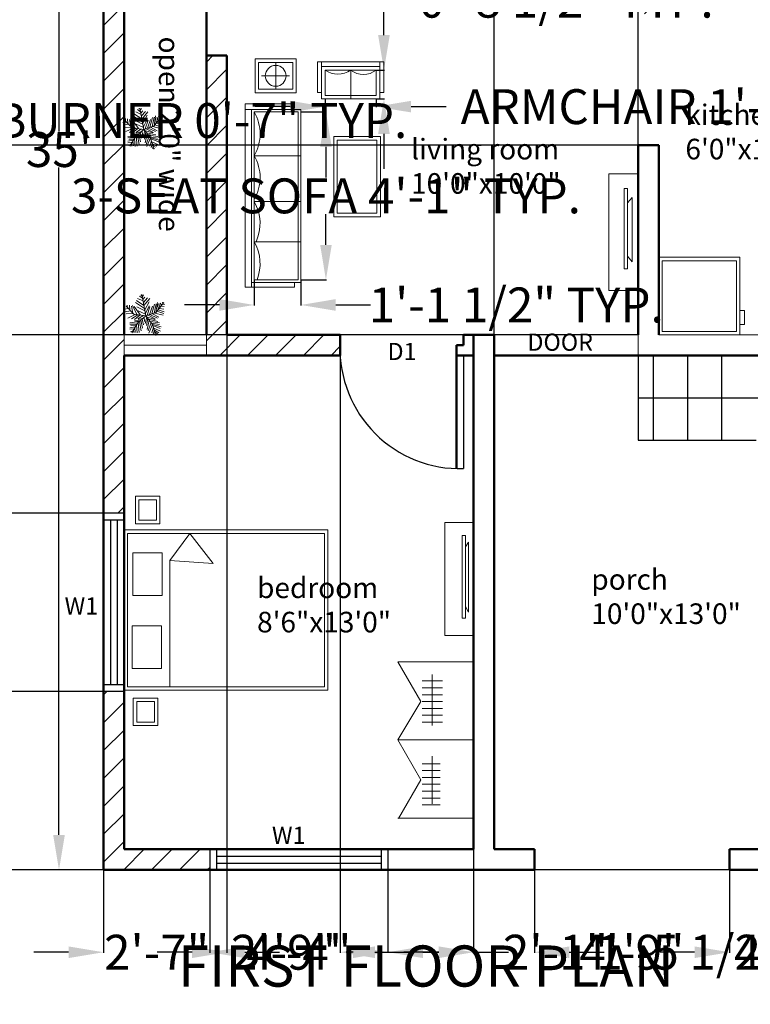
# Model space of a CAD drawing. Units: inches. Extents: x 21 to 3450, y 4 to 2137.
# Tile 12 of 14: x 3122 to 3335, y 1057 to 1344. Entities that reach past the tile are written whole.
import ezdxf

# ---------------------------------------------------------------- set-up
doc = ezdxf.new("R2010")
doc.units = ezdxf.units.IN
doc.header["$MEASUREMENT"] = 0
for name, color, linetype, lineweight in [('A-ANNO-DIMS', 2, 'Continuous', 18), ('A-ANNO-TEXT', 7, 'Continuous', 18), ('A-AREA-IDEN', 3, 'Continuous', 18), ('A-DOOR', 4, 'Continuous', 25), ('A-FLOR-FIXT', 9, 'Continuous', 18), ('A-FLOR-STRS', 2, 'Continuous', 25), ('A-FURN', 8, 'Continuous', 18), ('A-GLAZ', 3, 'Continuous', 25), ('A-WALL', 7, 'Continuous', 50), ('A-WALL-PATT', 8, 'Continuous', 13), ('L-PLNT', 94, 'Continuous', 13)]:
    doc.layers.add(name, color=color, linetype=linetype, lineweight=lineweight)
doc.styles.get("Standard").update_dxf_attribs({"font": 'arial.ttf'})
doc.dimstyles.get("Standard").update_dxf_attribs({"dimtxt": 10.18, "dimasz": 10.18, "dimexe": 0.18, "dimexo": 0.0625, "dimgap": 0.09, "dimtad": 0, "dimtih": 1, "dimtoh": 1, "dimdec": 0, "dimzin": 0, "dimdsep": 46, "dimlunit": 3, "dimtxsty": 'Standard', "dimcen": 0.09, "dimadec": 0, "dimazin": 0, "dimtfac": 1, "dimtdec": 0, "dimtofl": 0, "dimtmove": 0, "dimatfit": 3, "dimfxl": 1, "dimtolj": 1, "dimtzin": 0, "dimarcsym": 0})

# ---------------------------------------------------------------- blocks, each defined once
blk = doc.blocks.new('*U6')
for p, q in [((-8.737, 47.138), (-17.069, 52.711)), ((-10.186, 53.64), (-13.084, 55.962)), ((0, 0), (-10.5, 57)), ((-9.099, 51.782), (-6.563, 55.962)), ((-48.585, 21.131), (-49.309, 29.026)), ((-43.513, 28.561), (-42.427, 15.558)), ((-38.442, 26.239), (-34.819, 7.663)), ((-35.544, 28.097), (-24.314, 3.947)), ((-3.665, 19.273), (-27.574, 35.527)), ((-5.114, 28.097), (-24.676, 40.636)), ((-7.288, 39.707), (-21.778, 46.673)), ((-7.65, 43.423), (-2.578, 49.46)), ((-5.839, 35.992), (4.667, 48.067)), ((-5.114, 27.632), (10.463, 46.673)), ((-2.941, 16.486), (8.652, 37.85)), ((-1.129, 6.734), (9.014, 26.704)), ((10.101, 3.483), (17.708, 26.239)), ((16.259, 5.805), (23.142, 31.348)), ((22.055, 7.198), (27.489, 32.277)), ((27, 9), (48, 36)), ((27.127, 9.056), (31.112, 35.992)), ((31.836, 30.883), (32.561, 16.486)), ((35.096, 32.741), (37.27, 22.524)), ((38.719, 34.134), (41.979, 28.561)), ((43.791, 29.954), (51.036, 30.883)), ((44.153, 36.456), (45.239, 32.741)), ((-47.498, 19.737), (-55.83, 18.344)), ((-40.615, 13.7), (-55.105, 10.913)), ((-31.5, 4.5), (-52.5, 25.5)), ((-33.37, 6.269), (-52.207, 5.34)), ((-28.299, 3.483), (-47.86, -5.805)), ((-21.416, 3.018), (-38.079, -8.128)), ((0, 0), (-31.5, 4.5)), ((-14.533, 2.09), (-30.834, 25.31)), ((-15.982, 2.09), (-30.11, -9.521)), ((-24.314, 23.917), (-2.941, 13.7)), ((0, 0), (-22.5, -19.5)), ((-6.563, 1.161), (-21.416, -8.128)), ((-20.691, 13.7), (-1.129, 4.876)), ((0, 0), (27, 9)), ((0, 0), (18, -22.5)), ((3.942, 1.625), (11.187, 24.381)), ((6.478, 1.625), (26.04, -8.592)), ((11.187, 3.483), (30.749, -5.805)), ((18.07, 5.805), (35.096, -3.483)), ((24.229, 7.663), (46.688, 1.625)), ((29.662, 12.307), (48.137, 6.269)), ((33.285, 16.486), (48.862, 10.913)), ((36.183, 19.737), (48.137, 17.88)), ((40.53, 25.775), (48.862, 24.846)), ((-17.431, -15.094), (-42.789, -18.809)), ((-24.314, -21.596), (-42.427, -22.06)), ((-26.849, -26.24), (-40.253, -25.775)), ((-22.5, -19.5), (-37.5, -45)), ((-15.257, -12.772), (-30.11, -12.772)), ((-25.038, -23.918), (-22.865, -45.281)), ((-20.691, -18.345), (-17.793, -44.352)), ((-6.563, -5.805), (-19.967, -9.985)), ((-17.069, -15.094), (-12.721, -40.172)), ((-13.446, -11.378), (-8.737, -32.741)), ((-9.461, -8.592), (-6.201, -23.453)), ((-4.752, -3.483), (-3.665, -14.629)), ((2.493, -3.019), (-1.491, -20.202)), ((1.769, -2.555), (24.229, -9.521)), ((5.029, -6.27), (2.131, -25.775)), ((9.014, -11.378), (3.58, -35.992)), ((14.085, -16.951), (6.478, -40.172)), ((7.565, -9.056), (32.198, -14.629)), ((18.07, -22.524), (8.289, -45.745)), ((12.274, -15.094), (36.907, -18.809)), ((16.259, -19.738), (36.183, -22.989)), ((18, -22.5), (27, -52.5)), ((18.433, -22.524), (40.53, -29.026)), ((19.157, -25.311), (38.719, -33.206)), ((-28.299, -29.026), (-42.789, -31.348)), ((-30.834, -34.135), (-42.427, -35.528)), ((-34.457, -39.708), (-40.978, -42.494)), ((-32.646, -36.921), (-31.921, -44.352)), ((-29.023, -30.884), (-27.936, -43.887)), ((20.244, -30.419), (15.897, -44.816)), ((22.78, -37.85), (19.519, -48.532)), ((21.331, -32.741), (39.081, -40.636)), ((22.78, -38.314), (34.372, -44.816)), ((24.591, -45.745), (23.142, -50.854)), ((24.591, -43.423), (30.749, -47.603)), ((26.764, -49.925), (28.213, -50.854))]:
    blk.add_line(p, q)
blk = doc.blocks.new('*D10')
at = {"layer": 'A-ANNO-DIMS', "color": 0, "lineweight": -2, "transparency": 16777216}
for p, q in [((3146.55, 1515.83), (3133.43, 1515.83)), ((3133.61, 1505.65), (3133.61, 1311.09)), ((3133.61, 1105.95), (3133.61, 1300.51)), ((3329.19, 1095.77), (3133.43, 1095.77))]:
    blk.add_line(p, q, dxfattribs=at)
at = {"layer": 'A-ANNO-DIMS', "color": 0, "transparency": 16777216}
for points in [[(3131.91, 1505.65), (3135.31, 1505.65), (3133.61, 1515.83)], [(3131.91, 1105.95), (3135.31, 1105.95), (3133.61, 1095.77)]]:
    blk.add_solid(points, dxfattribs=at)
at = {"layer": 'Defpoints', "color": 0, "transparency": 16777216}
for p in [(3146.61, 1515.83), (3133.61, 1095.77), (3329.26, 1095.77)]:
    blk.add_point(p, dxfattribs=at)
at = {"layer": 'A-ANNO-DIMS', "color": 0, "transparency": 16777216, "insert": (3133.61, 1305.8), "char_height": 10.18, "attachment_point": 5}
blk.add_mtext("\\A1;35'", dxfattribs=at)
blk = doc.blocks.new('DOOR-35IN')
blk.add_line((36, 33.01), (36, 0.01))
blk.add_arc((35, 35.01), 35.01, 178.3634, 271.6366)
blk = doc.blocks.new('SOFA-3SEAT')
blk.add_line((0, 36.17), (13.59, 36.17))
blk.add_lwpolyline([(0, 48.92), (12.82, 48.92), (12.82, 0), (0, 0)], close=True)
for centre in [(-11.01, 42.54), (-11.01, 29.79)]:
    blk.add_arc(centre, 12.72, 329.9119, 30.0881)
blk = doc.blocks.new('ARMCHAIR')
blk.add_line((7.48, 8.43), (7.48, 0))
blk.add_lwpolyline([(0, 8.43), (14.95, 8.43), (14.95, 1), (0, 1)], close=True)
for centre, radius, start, end in [((3.74, 13.52), 6.31, 233.6798, 306.3202), ((11.21, 13.17), 6.03, 231.7288, 308.2712)]:
    blk.add_arc(centre, radius, start, end)
blk = doc.blocks.new('*D28')
at = {"layer": 'A-ANNO-DIMS', "color": 0, "lineweight": -2, "transparency": 16777216}
for p, q in [((3204.23, 1316.74), (3211.68, 1316.74)), ((3211.5, 1306.56), (3211.5, 1297.64)), ((3211.5, 1278), (3211.5, 1286.92)), ((3204.23, 1267.82), (3211.68, 1267.82))]:
    blk.add_line(p, q, dxfattribs=at)
at = {"layer": 'A-ANNO-DIMS', "color": 0, "transparency": 16777216}
for points in [[(3209.81, 1306.56), (3213.2, 1306.56), (3211.5, 1316.74)], [(3209.81, 1278), (3213.2, 1278), (3211.5, 1267.82)]]:
    blk.add_solid(points, dxfattribs=at)
at = {"layer": 'Defpoints', "color": 0, "transparency": 16777216}
for p in [(3204.17, 1316.74), (3211.5, 1316.74), (3204.17, 1267.82)]:
    blk.add_point(p, dxfattribs=at)
at = {"layer": 'A-ANNO-DIMS', "color": 0, "transparency": 16777216, "insert": (3211.5, 1292.28), "char_height": 10.18, "attachment_point": 5}
blk.add_mtext('\\A1;3-SEAT SOFA 4\'-1" TYP.', dxfattribs=at)
blk = doc.blocks.new('*D29')
at = {"layer": 'A-ANNO-DIMS', "color": 0, "lineweight": -2, "transparency": 16777216}
for p, q in [((3190.58, 1267.76), (3190.58, 1260.3)), ((3204.17, 1267.76), (3204.17, 1260.3)), ((3180.4, 1260.48), (3170.22, 1260.48)), ((3214.35, 1260.48), (3224.53, 1260.48))]:
    blk.add_line(p, q, dxfattribs=at)
at = {"layer": 'A-ANNO-DIMS', "color": 0, "transparency": 16777216}
for points in [[(3180.4, 1262.18), (3180.4, 1258.78), (3190.58, 1260.48)], [(3214.35, 1262.18), (3214.35, 1258.78), (3204.17, 1260.48)]]:
    blk.add_solid(points, dxfattribs=at)
at = {"layer": 'Defpoints', "color": 0, "transparency": 16777216}
for p in [(3190.58, 1267.82), (3204.17, 1267.82), (3204.17, 1260.48)]:
    blk.add_point(p, dxfattribs=at)
at = {"layer": 'A-ANNO-DIMS', "color": 0, "transparency": 16777216, "insert": (3267.02, 1260.48), "char_height": 10.18, "attachment_point": 5}
blk.add_mtext('\\A1;1\'-1 1/2" TYP.', dxfattribs=at)
blk = doc.blocks.new('*D30')
at = {"layer": 'A-ANNO-DIMS', "color": 0, "lineweight": -2, "transparency": 16777216}
for p, q in [((3201.06, 1318.3), (3190.88, 1318.3)), ((3211.24, 1320.48), (3211.24, 1318.12)), ((3226.19, 1320.48), (3226.19, 1318.12)), ((3236.37, 1318.3), (3246.55, 1318.3))]:
    blk.add_line(p, q, dxfattribs=at)
at = {"layer": 'A-ANNO-DIMS', "color": 0, "transparency": 16777216}
for points in [[(3201.06, 1320), (3201.06, 1316.61), (3211.24, 1318.3)], [(3236.37, 1320), (3236.37, 1316.61), (3226.19, 1318.3)]]:
    blk.add_solid(points, dxfattribs=at)
at = {"layer": 'Defpoints', "color": 0, "transparency": 16777216}
for p in [(3211.24, 1320.54), (3226.19, 1320.54), (3226.19, 1318.3)]:
    blk.add_point(p, dxfattribs=at)
at = {"layer": 'A-ANNO-DIMS', "color": 0, "transparency": 16777216, "insert": (3317.86, 1318.3), "char_height": 10.18, "attachment_point": 5}
blk.add_mtext('\\A1;ARMCHAIR 1\'-3" TYP.', dxfattribs=at)
blk = doc.blocks.new('*D31')
at = {"layer": 'A-ANNO-DIMS', "color": 0, "lineweight": -2, "transparency": 16777216}
for p, q in [((3228.43, 1339.16), (3228.43, 1349.34)), ((3228.43, 1349.34), (3238.61, 1349.34)), ((3226.25, 1328.98), (3228.61, 1328.98)), ((3226.25, 1320.54), (3228.61, 1320.54)), ((3228.43, 1310.36), (3228.43, 1300.18))]:
    blk.add_line(p, q, dxfattribs=at)
at = {"layer": 'A-ANNO-DIMS', "color": 0, "transparency": 16777216}
for points in [[(3226.74, 1339.16), (3230.13, 1339.16), (3228.43, 1328.98)], [(3226.74, 1310.36), (3230.13, 1310.36), (3228.43, 1320.54)]]:
    blk.add_solid(points, dxfattribs=at)
at = {"layer": 'Defpoints', "color": 0, "transparency": 16777216}
for p in [(3226.19, 1328.98), (3228.43, 1328.98), (3226.19, 1320.54)]:
    blk.add_point(p, dxfattribs=at)
at = {"layer": 'A-ANNO-DIMS', "color": 0, "transparency": 16777216, "insert": (3281.59, 1349.34), "char_height": 10.18, "attachment_point": 5}
blk.add_mtext('\\A1;0\'-8 1/2" TYP.', dxfattribs=at)
blk = doc.blocks.new('*D32')
at = {"layer": 'A-ANNO-DIMS', "color": 0, "lineweight": -2, "transparency": 16777216}
for p, q in [((3035.54, 1315.23), (3035.54, 1314.07)), ((3042.48, 1315.23), (3042.48, 1314.07)), ((3025.36, 1314.25), (3015.18, 1314.25)), ((3052.66, 1314.25), (3062.84, 1314.25))]:
    blk.add_line(p, q, dxfattribs=at)
at = {"layer": 'A-ANNO-DIMS', "color": 0, "transparency": 16777216}
for points in [[(3025.36, 1315.95), (3025.36, 1312.56), (3035.54, 1314.25)], [(3052.66, 1315.95), (3052.66, 1312.56), (3042.48, 1314.25)]]:
    blk.add_solid(points, dxfattribs=at)
at = {"layer": 'Defpoints', "color": 0, "transparency": 16777216}
for p in [(3035.54, 1315.29), (3042.48, 1315.29), (3042.48, 1314.25)]:
    blk.add_point(p, dxfattribs=at)
at = {"layer": 'A-ANNO-DIMS', "color": 0, "transparency": 16777216, "insert": (3152.02, 1314.25), "char_height": 10.18, "attachment_point": 5}
blk.add_mtext('\\A1;STOVE BURNER 0\'-7" TYP.', dxfattribs=at)
blk = doc.blocks.new('*D128')
at = {"layer": 'A-ANNO-DIMS', "color": 0, "lineweight": -2, "transparency": 16777216}
for p, q in [((3146.61, 1095.7), (3146.61, 1071.59)), ((3177.61, 1095.7), (3177.61, 1071.59)), ((3136.43, 1071.77), (3126.25, 1071.77)), ((3187.79, 1071.77), (3197.97, 1071.77))]:
    blk.add_line(p, q, dxfattribs=at)
at = {"layer": 'A-ANNO-DIMS', "color": 0, "transparency": 16777216}
for points in [[(3136.43, 1073.46), (3136.43, 1070.07), (3146.61, 1071.77)], [(3187.79, 1073.46), (3187.79, 1070.07), (3177.61, 1071.77)]]:
    blk.add_solid(points, dxfattribs=at)
at = {"layer": 'Defpoints', "color": 0, "transparency": 16777216}
for p in [(3146.61, 1095.77), (3177.61, 1095.77), (3177.61, 1071.77)]:
    blk.add_point(p, dxfattribs=at)
at = {"layer": 'A-ANNO-DIMS', "color": 0, "transparency": 16777216, "insert": (3162.11, 1071.77), "char_height": 10.18, "attachment_point": 5}
blk.add_mtext('\\A1;2\'-7"', dxfattribs=at)
blk = doc.blocks.new('*D129')
at = {"layer": 'A-ANNO-DIMS', "color": 0, "lineweight": -2, "transparency": 16777216}
for p, q in [((3177.61, 1095.7), (3177.61, 1071.59)), ((3229.61, 1095.7), (3229.61, 1071.59)), ((3187.79, 1071.77), (3189.79, 1071.77)), ((3219.43, 1071.77), (3217.44, 1071.77))]:
    blk.add_line(p, q, dxfattribs=at)
at = {"layer": 'A-ANNO-DIMS', "color": 0, "transparency": 16777216}
for points in [[(3187.79, 1073.46), (3187.79, 1070.07), (3177.61, 1071.77)], [(3219.43, 1073.46), (3219.43, 1070.07), (3229.61, 1071.77)]]:
    blk.add_solid(points, dxfattribs=at)
at = {"layer": 'Defpoints', "color": 0, "transparency": 16777216}
for p in [(3177.61, 1095.77), (3229.61, 1095.77), (3229.61, 1071.77)]:
    blk.add_point(p, dxfattribs=at)
at = {"layer": 'A-ANNO-DIMS', "color": 0, "transparency": 16777216, "insert": (3203.61, 1071.77), "char_height": 10.18, "attachment_point": 5}
blk.add_mtext('\\A1;4\'-4"', dxfattribs=at)
blk = doc.blocks.new('*D130')
at = {"layer": 'A-ANNO-DIMS', "color": 0, "lineweight": -2, "transparency": 16777216}
for p, q in [((3254.61, 1101.7), (3254.61, 1071.59)), ((3229.61, 1095.7), (3229.61, 1071.59)), ((3239.79, 1071.77), (3244.43, 1071.77)), ((3254.61, 1071.77), (3264.79, 1071.77))]:
    blk.add_line(p, q, dxfattribs=at)
at = {"layer": 'A-ANNO-DIMS', "color": 0, "transparency": 16777216}
for points in [[(3239.79, 1073.46), (3239.79, 1070.07), (3229.61, 1071.77)], [(3244.43, 1073.46), (3244.43, 1070.07), (3254.61, 1071.77)]]:
    blk.add_solid(points, dxfattribs=at)
at = {"layer": 'Defpoints', "color": 0, "transparency": 16777216}
for p in [(3254.61, 1101.77), (3229.61, 1095.77), (3254.61, 1071.77)]:
    blk.add_point(p, dxfattribs=at)
at = {"layer": 'A-ANNO-DIMS', "color": 0, "transparency": 16777216, "insert": (3278.5, 1071.77), "char_height": 10.18, "attachment_point": 5}
blk.add_mtext('\\A1;2\'-1"', dxfattribs=at)
blk = doc.blocks.new('*D131')
at = {"layer": 'A-ANNO-DIMS', "color": 0, "lineweight": -2, "transparency": 16777216}
for p, q in [((3254.61, 1101.7), (3254.61, 1071.59)), ((3272.34, 1095.7), (3272.34, 1071.59)), ((3244.43, 1071.77), (3234.25, 1071.77)), ((3282.52, 1071.77), (3292.7, 1071.77))]:
    blk.add_line(p, q, dxfattribs=at)
at = {"layer": 'A-ANNO-DIMS', "color": 0, "transparency": 16777216}
for points in [[(3244.43, 1073.46), (3244.43, 1070.07), (3254.61, 1071.77)], [(3282.52, 1073.46), (3282.52, 1070.07), (3272.34, 1071.77)]]:
    blk.add_solid(points, dxfattribs=at)
at = {"layer": 'Defpoints', "color": 0, "transparency": 16777216}
for p in [(3254.61, 1101.77), (3272.34, 1095.77), (3272.34, 1071.77)]:
    blk.add_point(p, dxfattribs=at)
at = {"layer": 'A-ANNO-DIMS', "color": 0, "transparency": 16777216, "insert": (3317.7, 1071.77), "char_height": 10.18, "attachment_point": 5}
blk.add_mtext('\\A1;1\'-5 1/2"', dxfattribs=at)
blk = doc.blocks.new('*D132')
at = {"layer": 'A-ANNO-DIMS', "color": 0, "lineweight": -2, "transparency": 16777216}
for p, q in [((3272.34, 1095.7), (3272.34, 1071.59)), ((3329.26, 1095.7), (3329.26, 1071.59)), ((3282.52, 1071.77), (3286.97, 1071.77)), ((3319.08, 1071.77), (3314.62, 1071.77))]:
    blk.add_line(p, q, dxfattribs=at)
at = {"layer": 'A-ANNO-DIMS', "color": 0, "transparency": 16777216}
for points in [[(3282.52, 1073.46), (3282.52, 1070.07), (3272.34, 1071.77)], [(3319.08, 1073.46), (3319.08, 1070.07), (3329.26, 1071.77)]]:
    blk.add_solid(points, dxfattribs=at)
at = {"layer": 'Defpoints', "color": 0, "transparency": 16777216}
for p in [(3272.34, 1095.77), (3329.26, 1095.77), (3329.26, 1071.77)]:
    blk.add_point(p, dxfattribs=at)
at = {"layer": 'A-ANNO-DIMS', "color": 0, "transparency": 16777216, "insert": (3300.8, 1071.77), "char_height": 10.18, "attachment_point": 5}
blk.add_mtext('\\A1;4\'-9"', dxfattribs=at)
blk = doc.blocks.new('*D133')
at = {"layer": 'A-ANNO-DIMS', "color": 0, "lineweight": -2, "transparency": 16777216}
for p, q in [((3329.26, 1095.7), (3329.26, 1071.59)), ((3386.61, 1095.7), (3386.61, 1071.59)), ((3319.08, 1071.77), (3308.9, 1071.77)), ((3396.79, 1071.77), (3406.97, 1071.77))]:
    blk.add_line(p, q, dxfattribs=at)
at = {"layer": 'A-ANNO-DIMS', "color": 0, "transparency": 16777216}
for points in [[(3319.08, 1073.46), (3319.08, 1070.07), (3329.26, 1071.77)], [(3396.79, 1073.46), (3396.79, 1070.07), (3386.61, 1071.77)]]:
    blk.add_solid(points, dxfattribs=at)
at = {"layer": 'Defpoints', "color": 0, "transparency": 16777216}
for p in [(3329.26, 1095.77), (3386.61, 1095.77), (3386.61, 1071.77)]:
    blk.add_point(p, dxfattribs=at)
at = {"layer": 'A-ANNO-DIMS', "color": 0, "transparency": 16777216, "insert": (3357.93, 1071.77), "char_height": 10.18, "attachment_point": 5}
blk.add_mtext('\\A1;4\'-9 1/2"', dxfattribs=at)
blk = doc.blocks.new('*D141')
at = {"layer": 'A-ANNO-DIMS', "color": 0, "lineweight": -2, "transparency": 16777216}
for p, q in [((3146.55, 1147.77), (3068.43, 1147.77)), ((3068.61, 1137.59), (3068.61, 1126.95)), ((3068.61, 1105.95), (3068.61, 1116.59)), ((3146.55, 1095.77), (3068.43, 1095.77))]:
    blk.add_line(p, q, dxfattribs=at)
at = {"layer": 'A-ANNO-DIMS', "color": 0, "transparency": 16777216}
for points in [[(3066.91, 1137.59), (3070.31, 1137.59), (3068.61, 1147.77)], [(3066.91, 1105.95), (3070.31, 1105.95), (3068.61, 1095.77)]]:
    blk.add_solid(points, dxfattribs=at)
at = {"layer": 'Defpoints', "color": 0, "transparency": 16777216}
for p in [(3068.61, 1147.77), (3146.61, 1147.77), (3146.61, 1095.77)]:
    blk.add_point(p, dxfattribs=at)
at = {"layer": 'A-ANNO-DIMS', "color": 0, "transparency": 16777216, "insert": (3068.61, 1121.77), "char_height": 10.18, "attachment_point": 5}
blk.add_mtext('\\A1;4\'-4"', dxfattribs=at)
blk = doc.blocks.new('*D142')
at = {"layer": 'A-ANNO-DIMS', "color": 0, "lineweight": -2, "transparency": 16777216}
for p, q in [((3146.55, 1199.77), (3068.43, 1199.77)), ((3068.61, 1189.59), (3068.61, 1178.95)), ((3068.61, 1157.95), (3068.61, 1168.59)), ((3146.55, 1147.77), (3068.43, 1147.77))]:
    blk.add_line(p, q, dxfattribs=at)
at = {"layer": 'A-ANNO-DIMS', "color": 0, "transparency": 16777216}
for points in [[(3066.91, 1189.59), (3070.31, 1189.59), (3068.61, 1199.77)], [(3066.91, 1157.95), (3070.31, 1157.95), (3068.61, 1147.77)]]:
    blk.add_solid(points, dxfattribs=at)
at = {"layer": 'Defpoints', "color": 0, "transparency": 16777216}
for p in [(3068.61, 1199.77), (3146.61, 1199.77), (3146.61, 1147.77)]:
    blk.add_point(p, dxfattribs=at)
at = {"layer": 'A-ANNO-DIMS', "color": 0, "transparency": 16777216, "insert": (3068.61, 1173.77), "char_height": 10.18, "attachment_point": 5}
blk.add_mtext('\\A1;4\'-4"', dxfattribs=at)
blk = doc.blocks.new('*D144')
at = {"layer": 'A-ANNO-DIMS', "color": 0, "lineweight": -2, "transparency": 16777216}
for p, q in [((3182.61, 1251.7), (3182.61, 1071.59)), ((3215.61, 1251.7), (3215.61, 1071.59)), ((3172.43, 1071.77), (3162.25, 1071.77)), ((3225.79, 1071.77), (3235.97, 1071.77))]:
    blk.add_line(p, q, dxfattribs=at)
at = {"layer": 'A-ANNO-DIMS', "color": 0, "transparency": 16777216}
for points in [[(3172.43, 1073.46), (3172.43, 1070.07), (3182.61, 1071.77)], [(3225.79, 1073.46), (3225.79, 1070.07), (3215.61, 1071.77)]]:
    blk.add_solid(points, dxfattribs=at)
at = {"layer": 'Defpoints', "color": 0, "transparency": 16777216}
for p in [(3182.61, 1251.77), (3215.61, 1251.77), (3215.61, 1071.77)]:
    blk.add_point(p, dxfattribs=at)
at = {"layer": 'A-ANNO-DIMS', "color": 0, "transparency": 16777216, "insert": (3199.11, 1071.77), "char_height": 10.18, "attachment_point": 5}
blk.add_mtext('\\A1;2\'-9"', dxfattribs=at)
blk = doc.blocks.new('*D145')
at = {"layer": 'A-ANNO-DIMS', "color": 0, "lineweight": -2, "transparency": 16777216}
for p, q in [((3250.43, 1547.93), (3240.25, 1547.93)), ((3260.61, 1251.83), (3260.61, 1548.11)), ((3302.61, 1251.83), (3302.61, 1548.11)), ((3312.79, 1547.93), (3322.97, 1547.93))]:
    blk.add_line(p, q, dxfattribs=at)
at = {"layer": 'A-ANNO-DIMS', "color": 0, "transparency": 16777216}
for points in [[(3250.43, 1549.63), (3250.43, 1546.23), (3260.61, 1547.93)], [(3312.79, 1549.63), (3312.79, 1546.23), (3302.61, 1547.93)]]:
    blk.add_solid(points, dxfattribs=at)
at = {"layer": 'Defpoints', "color": 0, "transparency": 16777216}
for p in [(3302.61, 1547.93), (3260.61, 1251.77), (3302.61, 1251.77)]:
    blk.add_point(p, dxfattribs=at)
at = {"layer": 'A-ANNO-DIMS', "color": 0, "transparency": 16777216, "insert": (3281.61, 1547.93), "char_height": 10.18, "attachment_point": 5}
blk.add_mtext('\\A1;3\'-6"', dxfattribs=at)
blk = doc.blocks.new('*D147')
at = {"layer": 'A-ANNO-DIMS', "color": 0, "lineweight": -2, "transparency": 16777216}
for p, q in [((3302.55, 1307.09), (3068.43, 1307.09)), ((3068.61, 1296.91), (3068.61, 1284.78)), ((3068.61, 1261.95), (3068.61, 1274.08)), ((3302.55, 1251.77), (3068.43, 1251.77))]:
    blk.add_line(p, q, dxfattribs=at)
at = {"layer": 'A-ANNO-DIMS', "color": 0, "transparency": 16777216}
for points in [[(3066.91, 1296.91), (3070.31, 1296.91), (3068.61, 1307.09)], [(3066.91, 1261.95), (3070.31, 1261.95), (3068.61, 1251.77)]]:
    blk.add_solid(points, dxfattribs=at)
at = {"layer": 'Defpoints', "color": 0, "transparency": 16777216}
for p in [(3068.61, 1307.09), (3302.61, 1307.09), (3302.61, 1251.77)]:
    blk.add_point(p, dxfattribs=at)
at = {"layer": 'A-ANNO-DIMS', "color": 0, "transparency": 16777216, "insert": (3068.61, 1279.43), "char_height": 10.18, "attachment_point": 5}
blk.add_mtext('\\A1;4\'-7 1/2"', dxfattribs=at)

msp = doc.modelspace()

# ---------------------------------------------------------------- hatches: boundary and pattern name
at = {"layer": 'A-WALL-PATT'}
h = msp.add_hatch(dxfattribs=at)
h.set_pattern_fill('ANSI31', color=256, scale=46)
h.set_pattern_definition([(45, (297.6833, 160.0466), (-4.065864, 4.065864), [])])
h.paths.add_polyline_path([(3281.11, 1515.77), (3146.61, 1515.77), (3146.61, 1199.77), (3152.61, 1199.77), (3152.61, 1245.77), (3152.61, 1251.77), (3152.61, 1371.77), (3152.61, 1377.77), (3152.61, 1461.77), (3176.11, 1461.77), (3176.11, 1467.77), (3152.61, 1467.77), (3152.61, 1509.77), (3227.61, 1509.77), (3233.61, 1509.77), (3281.11, 1509.77)])
h.paths.add_polyline_path([(3386.61, 1515.77), (3333.11, 1515.77), (3333.11, 1509.77), (3380.61, 1509.77), (3380.61, 1469.33, -0.065004), (3380.75, 1468.31), (3380.75, 1431.5, -0.065004), (3380.61, 1430.47), (3380.61, 1377.77), (3272.1, 1377.77), (3272.1, 1374.77), (3274.1, 1374.77), (3274.1, 1371.77), (3302.61, 1371.77), (3302.61, 1345.32), (3308.61, 1345.32), (3308.61, 1371.77), (3380.61, 1371.77), (3380.61, 1337.77), (3386.61, 1337.77)])
h.paths.add_polyline_path([(3215.61, 1248.77), (3215.61, 1251.77), (3182.61, 1251.77), (3182.61, 1333.19), (3176.61, 1333.19), (3176.61, 1251.77), (3176.61, 1245.77), (3215.61, 1245.77), (3215.61, 1246.77, -0.014283)], flags=17)
h.paths.add_polyline_path([(3177.61, 1101.77), (3152.61, 1101.77), (3152.61, 1147.77), (3146.61, 1147.77), (3146.61, 1095.77), (3177.61, 1095.77)])
h.paths.add_polyline_path([(3241.1, 1377.77), (3233.61, 1377.77), (3227.61, 1377.77), (3176.61, 1377.77), (3176.61, 1371.77), (3182.61, 1371.77), (3233.61, 1371.77), (3241.1, 1371.77)], flags=17)
h.paths.add_polyline_path([(3233.61, 1467.77), (3227.61, 1467.77), (3204.11, 1467.77), (3204.11, 1461.77), (3227.61, 1461.77), (3227.61, 1410.77), (3228.61, 1410.77, -0.017236), (3230.61, 1410.77), (3233.61, 1410.77), (3233.61, 1461.77)], flags=17)

# ---------------------------------------------------------------- linework, layer by layer
at = {"layer": 'A-FLOR-FIXT'}
for points in [[(3308.61, 1251.77), (3308.61, 1251.77), (3332.3, 1251.77), (3332.3, 1251.77), (3332.3, 1274.37), (3332.3, 1274.37), (3308.61, 1274.37), (3308.61, 1274.37)], [(3309.61, 1252.77), (3331.3, 1252.77), (3331.3, 1273.37), (3309.61, 1273.37)], [(3332.3, 1254.75), (3332.3, 1254.75), (3333.62, 1254.75), (3333.62, 1254.75), (3333.62, 1258.9), (3333.62, 1258.9), (3332.3, 1258.9), (3332.3, 1258.9)]]:
    msp.add_lwpolyline(points, close=True, dxfattribs=at)
at = {"layer": 'A-FLOR-STRS'}
for p, q in [((3302.61, 1245.77), (3302.61, 1221.07)), ((3307.06, 1221.07), (3307.06, 1245.77)), ((3317.06, 1221.07), (3317.06, 1245.77)), ((3327.06, 1221.07), (3327.06, 1245.77)), ((3302.61, 1233.42), (3361.91, 1233.42)), ((3302.61, 1221.07), (3337.06, 1221.07))]:
    msp.add_line(p, q, dxfattribs=at)
at = {"layer": 'A-FURN'}
for p, q in [((3196.84, 1331.21), (3196.84, 1323.35)), ((3192.72, 1327.28), (3200.89, 1327.29)), ((3190.58, 1290.62), (3204.17, 1290.62)), ((3299.51, 1290.23), (3300.88, 1291.78)), ((3300.88, 1291.78), (3300.88, 1273.1)), ((3190.58, 1278.86), (3204.17, 1278.86)), ((3300.88, 1273.1), (3299.51, 1274.73)), ((3189.76, 1265.68), (3187.91, 1265.68)), ((3152.61, 1251.77), (3176.61, 1251.77)), ((3152.61, 1251.77), (3152.61, 1245.77)), ((3176.61, 1251.77), (3176.61, 1245.77)), ((3302.61, 1251.77), (3302.61, 1245.77)), ((3308.61, 1251.77), (3380.61, 1251.77)), ((3176.61, 1248.77), (3152.61, 1248.77)), ((3165.94, 1186.01), (3171.81, 1193.88)), ((3171.81, 1193.88), (3178.59, 1185.14)), ((3252.22, 1189.96), (3253.07, 1191.28)), ((3253.07, 1191.28), (3253.07, 1170.88)), ((3165.94, 1149.18), (3165.94, 1186.01)), ((3178.59, 1185.14), (3165.94, 1186.01)), ((3253.07, 1170.88), (3252.22, 1172.59)), ((3232.44, 1156.46), (3239.15, 1144.83)), ((3242.48, 1152.74), (3242.48, 1137.91)), ((3239.58, 1150.85), (3245.5, 1150.85)), ((3239.58, 1148.85), (3245.5, 1148.85)), ((3239.58, 1146.85), (3245.5, 1146.85)), ((3239.15, 1144.83), (3232.44, 1133.67)), ((3239.58, 1144.85), (3245.5, 1144.85)), ((3239.58, 1142.85), (3245.5, 1142.85)), ((3239.58, 1140.85), (3245.5, 1140.85)), ((3239.58, 1138.85), (3245.5, 1138.85)), ((3232.44, 1133.67), (3254.61, 1133.67)), ((3232.44, 1133.67), (3239.17, 1122.02)), ((3242.48, 1128.93), (3242.48, 1115.01)), ((3239.63, 1126.73), (3244.85, 1126.73)), ((3239.63, 1124.73), (3244.85, 1124.73)), ((3239.63, 1122.73), (3244.85, 1122.73)), ((3239.17, 1122.02), (3232.67, 1110.76)), ((3239.63, 1120.73), (3244.85, 1120.73)), ((3239.63, 1118.73), (3244.85, 1118.73)), ((3239.63, 1116.73), (3244.85, 1116.73)), ((3239.63, 1114.73), (3244.85, 1114.73))]:
    msp.add_line(p, q, dxfattribs=at)
for points in [[(3190.87, 1332.21), (3202.81, 1332.21), (3202.81, 1322.35), (3190.87, 1322.35)], [(3191.87, 1331.21), (3191.87, 1331.21), (3201.81, 1331.21), (3201.81, 1331.21), (3201.81, 1323.35), (3201.81, 1323.35), (3191.87, 1323.35), (3191.87, 1323.35)], [(3210.24, 1322.47), (3210.24, 1322.47), (3209.06, 1322.47), (3209.06, 1322.47), (3209.06, 1331.35), (3209.06, 1331.35), (3210.24, 1331.35), (3210.24, 1331.35)], [(3210.24, 1331.35), (3210.24, 1331.35), (3227.19, 1331.35), (3227.19, 1331.35), (3227.19, 1329.98), (3227.19, 1329.98), (3210.24, 1329.98), (3210.24, 1329.98)], [(3210.24, 1329.98), (3210.24, 1329.98), (3227.19, 1329.98), (3227.19, 1329.98), (3227.19, 1320.54), (3227.19, 1320.54), (3210.24, 1320.54), (3210.24, 1320.54)], [(3228.37, 1322.47), (3228.37, 1322.47), (3227.19, 1322.47), (3227.19, 1322.47), (3227.19, 1331.35), (3227.19, 1331.35), (3228.37, 1331.35), (3228.37, 1331.35)], [(3201.95, 1317.51), (3201.95, 1317.51), (3187.91, 1317.51), (3187.91, 1317.51), (3187.91, 1319.14), (3187.91, 1319.14), (3201.95, 1319.14), (3201.95, 1319.14)], [(3189.81, 1317.51), (3189.81, 1317.51), (3204.17, 1317.51), (3204.17, 1317.51), (3204.17, 1267.06), (3204.17, 1267.06), (3189.81, 1267.06), (3189.81, 1267.06)], [(3213.76, 1309.56), (3213.76, 1309.56), (3227.38, 1309.56), (3227.38, 1309.56), (3227.38, 1286.21), (3227.38, 1286.21), (3213.76, 1286.21), (3213.76, 1286.21)], [(3214.76, 1308.56), (3226.38, 1308.56), (3226.38, 1287.21), (3214.76, 1287.21)], [(3302.61, 1298.68), (3302.61, 1298.68), (3294.04, 1298.68), (3294.04, 1298.68), (3294.04, 1264.68), (3294.04, 1264.68), (3302.61, 1264.68), (3302.61, 1264.68)], [(3299.51, 1294.43), (3299.51, 1294.43), (3298.57, 1294.43), (3298.57, 1294.43), (3298.57, 1271.04), (3298.57, 1271.04), (3299.51, 1271.04), (3299.51, 1271.04)], [(3189.76, 1267.06), (3189.76, 1267.06), (3202.29, 1267.06), (3202.29, 1267.06), (3202.29, 1265.68), (3202.29, 1265.68), (3189.76, 1265.68), (3189.76, 1265.68)], [(3155.9, 1204.69), (3155.9, 1204.69), (3163.05, 1204.69), (3163.05, 1204.69), (3163.05, 1196.71), (3163.05, 1196.71), (3155.9, 1196.71), (3155.9, 1196.71)], [(3156.9, 1203.69), (3162.05, 1203.69), (3162.05, 1197.71), (3156.9, 1197.71)], [(3152.61, 1194.88), (3152.61, 1194.88), (3212.07, 1194.88), (3212.07, 1194.88), (3212.07, 1148.18), (3212.07, 1148.18), (3152.61, 1148.18), (3152.61, 1148.18)], [(3254.61, 1197.04), (3254.61, 1197.04), (3246.22, 1197.04), (3246.22, 1197.04), (3246.22, 1164.15), (3246.22, 1164.15), (3254.61, 1164.15), (3254.61, 1164.15)], [(3153.61, 1193.88), (3211.07, 1193.88), (3211.07, 1149.18), (3153.61, 1149.18)], [(3251.26, 1193.22), (3251.26, 1193.22), (3252.22, 1193.22), (3252.22, 1193.22), (3252.22, 1169.12), (3252.22, 1169.12), (3251.26, 1169.12), (3251.26, 1169.12)], [(3155.17, 1188.19), (3155.17, 1188.19), (3163.76, 1188.19), (3163.76, 1188.19), (3163.76, 1175.74), (3163.76, 1175.74), (3155.17, 1175.74), (3155.17, 1175.74)], [(3154.97, 1166.9), (3154.97, 1166.9), (3163.56, 1166.9), (3163.56, 1166.9), (3163.56, 1154.45), (3163.56, 1154.45), (3154.97, 1154.45), (3154.97, 1154.45)], [(3155.29, 1145.85), (3155.29, 1145.85), (3162.45, 1145.85), (3162.45, 1145.85), (3162.45, 1137.86), (3162.45, 1137.86), (3155.29, 1137.86), (3155.29, 1137.86)], [(3156.29, 1144.85), (3161.45, 1144.85), (3161.45, 1138.86), (3156.29, 1138.86)]]:
    msp.add_lwpolyline(points, close=True, dxfattribs=at)
for points in [[(3187.91, 1265.68), (3187.91, 1317.51), (3187.91, 1317.51), (3189.76, 1317.51), (3189.76, 1317.51), (3189.76, 1265.68)], [(3232.44, 1110.89), (3232.44, 1110.89), (3254.61, 1110.89), (3254.61, 1110.89), (3254.61, 1156.46), (3254.61, 1156.46), (3232.44, 1156.46), (3232.44, 1156.46)]]:
    msp.add_lwpolyline(points, dxfattribs=at)
msp.add_circle((3196.84, 1327.28), 3.03, dxfattribs=at)
for centre, start, end in [((3179.57, 1310.36), 323.186, 323.6288), ((3179.57, 1284.24), 334.9772, 30.0881), ((3179.57, 1272.49), 338.4844, 30.0881)]:
    msp.add_arc(centre, 12.72, start, end, dxfattribs=at)
at = {"layer": 'A-GLAZ'}
for p, q in [((3152.61, 1199.77), (3146.61, 1199.77)), ((3152.61, 1197.77), (3146.61, 1197.77)), ((3148.61, 1197.77), (3148.61, 1149.77)), ((3150.61, 1197.77), (3150.61, 1149.77)), ((3152.61, 1149.77), (3146.61, 1149.77)), ((3152.61, 1147.77), (3146.61, 1147.77)), ((3177.61, 1101.77), (3177.61, 1095.77)), ((3179.61, 1101.77), (3179.61, 1095.77)), ((3179.61, 1099.77), (3227.61, 1099.77)), ((3227.61, 1101.77), (3227.61, 1095.77)), ((3229.61, 1101.77), (3229.61, 1095.77)), ((3179.61, 1097.77), (3227.61, 1097.77))]:
    msp.add_line(p, q, dxfattribs=at)
at = {"layer": 'A-WALL'}
for p, q in [((3146.61, 1095.77), (3146.61, 1515.77)), ((3152.61, 1251.77), (3152.61, 1371.77)), ((3176.61, 1371.77), (3176.61, 1251.77)), ((3176.61, 1333.19), (3182.61, 1333.19)), ((3182.61, 1333.19), (3182.61, 1251.77)), ((3302.61, 1307.09), (3302.61, 1251.77)), ((3302.61, 1307.09), (3308.61, 1307.09)), ((3308.61, 1307.09), (3308.61, 1251.77)), ((3182.61, 1251.77), (3215.61, 1251.77)), ((3215.61, 1245.77), (3215.61, 1251.77)), ((3251.61, 1251.77), (3260.61, 1251.77)), ((3251.61, 1248.77), (3251.61, 1251.77)), ((3254.61, 1245.77), (3254.61, 1251.77)), ((3260.61, 1245.77), (3260.61, 1251.77)), ((3249.61, 1248.77), (3249.61, 1212.77)), ((3249.61, 1248.77), (3251.61, 1248.77)), ((3152.61, 1101.77), (3152.61, 1245.77)), ((3152.61, 1245.77), (3215.65, 1245.77)), ((3249.61, 1245.77), (3254.61, 1245.77)), ((3254.61, 1101.77), (3254.61, 1245.77)), ((3260.61, 1101.77), (3260.61, 1245.77)), ((3260.61, 1245.77), (3380.61, 1245.77)), ((3254.61, 1101.77), (3152.61, 1101.77)), ((3272.34, 1101.77), (3260.61, 1101.77)), ((3272.34, 1101.77), (3272.34, 1095.77)), ((3380.61, 1101.77), (3329.26, 1101.77)), ((3329.26, 1101.77), (3329.26, 1095.77)), ((3272.34, 1095.77), (3146.61, 1095.77)), ((3386.61, 1095.77), (3329.26, 1095.77))]:
    msp.add_line(p, q, dxfattribs=at)

# ---------------------------------------------------------------- block references
at = {"layer": 'A-DOOR'}
msp.add_blockref('DOOR-35IN', (3215.61, 1212.76), dxfattribs=at)
at = {"layer": 'A-FURN'}
for name, p in [('ARMCHAIR', (3211.24, 1320.54)), ('SOFA-3SEAT', (3190.58, 1267.82))]:
    msp.add_blockref(name, p, dxfattribs=at)
at = {"layer": 'L-PLNT', "xscale": 0.1095009231923873, "yscale": 0.1095009231923873, "zscale": 0.1095009231923873}
for p in [(3158.37, 1311.66), (3158.94, 1257.29)]:
    msp.add_blockref('*U6', p, dxfattribs=at)

# ---------------------------------------------------------------- texts
at = {"layer": 'A-ANNO-TEXT', "insert": (3168.76, 1338.73), "char_height": 6, "attachment_point": 1, "rotation": 270}
msp.add_mtext_dynamic_manual_height_columns('open 2\'0" wide', width=84.0083, gutter_width=1, heights=[0], dxfattribs=at)
at = {"layer": 'A-ANNO-TEXT', "attachment_point": 1}
for s, width, insert, char_height in [('DOOR', 14.628, (3270.28, 1252.12), 5), ('D1', 14.628, (3229.47, 1249.42), 5), ('W1', 14.628, (3135.26, 1175.21), 5), ('W1', 14.628, (3195.76, 1108.34), 5), ('FIRST FLOOR PLAN', 189.6067, (3168.31, 1073.74), 12)]:
    msp.add_mtext_dynamic_manual_height_columns(s, width=width, gutter_width=1, heights=[0], dxfattribs=dict(at, insert=insert, char_height=char_height))
at = {"layer": 'A-AREA-IDEN', "char_height": 6, "attachment_point": 1}
for s, insert in [('kitchen\\P6\'0"x10\'0"', (3316.4, 1318.93)), ('living room\\P10\'0"x10\'0"', (3236.35, 1308.91)), ('porch\\P10\'0"x13\'0"', (3288.94, 1183.47)), ('bedroom\\P8\'6"x13\'0"', (3191.41, 1181.02))]:
    msp.add_mtext_dynamic_manual_height_columns(s, width=84.0083, gutter_width=1, heights=[0], dxfattribs=dict(at, insert=insert))

# ---------------------------------------------------------------- dimensions: what is measured, and where the dimension line sits
at = {"layer": 'A-ANNO-DIMS'}
for base, p1, p2, picture, middle in [((3302.61, 1547.93), (3260.61, 1251.77), (3302.61, 1251.77), '*D145', (3281.61, 1547.93)), ((3215.61, 1071.77), (3182.61, 1251.77), (3215.61, 1251.77), '*D144', (3199.11, 1071.77)), ((3254.61, 1071.77), (3229.61, 1095.77), (3254.61, 1101.77), '*D130', (3278.5, 1071.77)), ((3272.34, 1071.77), (3254.61, 1101.77), (3272.34, 1095.77), '*D131', (3317.7, 1071.77)), ((3177.61, 1071.77), (3146.61, 1095.77), (3177.61, 1095.77), '*D128', (3162.11, 1071.77)), ((3229.61, 1071.77), (3177.61, 1095.77), (3229.61, 1095.77), '*D129', (3203.61, 1071.77)), ((3329.26, 1071.77), (3272.34, 1095.77), (3329.26, 1095.77), '*D132', (3300.8, 1071.77)), ((3386.611, 1071.7664), (3329.2573, 1095.7664), (3386.611, 1095.7664), '*D133', (3357.9341, 1071.7664))]:
    dim = msp.add_linear_dim(base=base, p1=p1, p2=p2, dimstyle='Standard', override={"dimdec": 1, "dimlfac": 1, "dimrnd": 0, "dimzin": 1, "dimdsep": 46, "dimlunit": 4, "dimfrac": 2}, dxfattribs=at)
    dim.commit()
    dim.dimension.update_dxf_attribs({"geometry": picture, "text_midpoint": middle})
for base, p1, p2, override, picture, middle in [((3133.61, 1095.77), (3146.61, 1515.83), (3329.26, 1095.77), {"dimclrd": 0, "dimclre": 0, "dimclrt": 0}, '*D10', (3133.61, 1305.8)), ((3068.61, 1307.09), (3302.61, 1251.77), (3302.61, 1307.09), {"dimdec": 1, "dimlfac": 1, "dimrnd": 0, "dimzin": 1, "dimdsep": 46, "dimlunit": 4, "dimfrac": 2}, '*D147', (3068.61, 1279.43)), ((3068.61, 1199.77), (3146.61, 1147.77), (3146.61, 1199.77), {"dimdec": 1, "dimlfac": 1, "dimrnd": 0, "dimzin": 1, "dimdsep": 46, "dimlunit": 4, "dimfrac": 2}, '*D142', (3068.61, 1173.77)), ((3068.61, 1147.77), (3146.61, 1095.77), (3146.61, 1147.77), {"dimdec": 1, "dimlfac": 1, "dimrnd": 0, "dimzin": 1, "dimdsep": 46, "dimlunit": 4, "dimfrac": 2}, '*D141', (3068.61, 1121.77))]:
    dim = msp.add_linear_dim(base=base, p1=p1, p2=p2, angle=90, dimstyle='Standard', override=override, dxfattribs=at)
    dim.commit()
    dim.dimension.update_dxf_attribs({"geometry": picture, "text_midpoint": middle})
for base, p1, p2, text, picture, middle in [((3228.43, 1328.98), (3226.19, 1320.54), (3226.19, 1328.98), '<> TYP.', '*D31', (3281.59, 1349.34)), ((3211.5, 1316.74), (3204.17, 1267.82), (3204.17, 1316.74), '3-SEAT SOFA <> TYP.', '*D28', (3211.5, 1292.28))]:
    dim = msp.add_linear_dim(base=base, p1=p1, p2=p2, angle=90, text=text, dimstyle='Standard', override={"dimdec": 1, "dimrnd": 0, "dimzin": 1, "dimlunit": 4, "dimfrac": 2}, dxfattribs=at)
    dim.commit()
    dim.dimension.update_dxf_attribs({"geometry": picture, "text_midpoint": middle})
for base, p1, p2, text, picture, middle in [((3042.48, 1314.25), (3035.54, 1315.29), (3042.48, 1315.29), 'STOVE BURNER <> TYP.', '*D32', (3152.02, 1314.25)), ((3226.1906, 1318.3019), (3211.2391, 1320.5447), (3226.1906, 1320.5447), 'ARMCHAIR <> TYP.', '*D30', (3317.8624, 1318.3019)), ((3204.17, 1260.48), (3190.58, 1267.82), (3204.17, 1267.82), '<> TYP.', '*D29', (3267.02, 1260.48))]:
    dim = msp.add_linear_dim(base=base, p1=p1, p2=p2, text=text, dimstyle='Standard', override={"dimdec": 1, "dimrnd": 0, "dimzin": 1, "dimlunit": 4, "dimfrac": 2}, dxfattribs=at)
    dim.commit()
    dim.dimension.update_dxf_attribs({"geometry": picture, "text_midpoint": middle})

doc.saveas('drawing.dxf')
